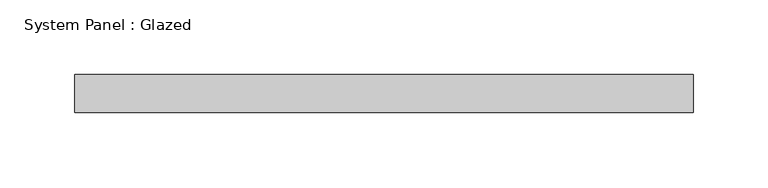
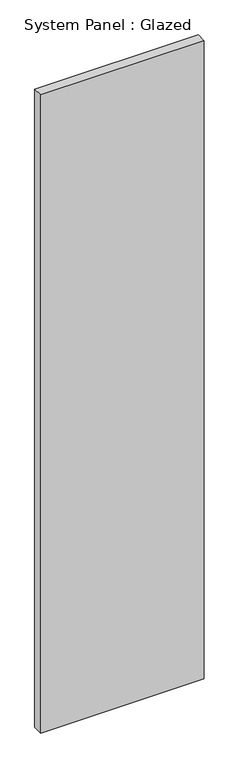
"""IFC4 building model written with IfcOpenShell, lengths in millimetres: plate geometry, System Panel : Glazed."""

from ifc_helpers import new_model, si_unit, origin, origin_with_axes, place, context, project, spatial, polyline, outline, extrude, source, transform, mapped, element, save


def system_panel_glazed_c73a426b(model_context):
    return source(origin(), model_context, "Body", "SweptSolid", [
        extrude(outline(polyline([(206.375, 19.05), (-206.375, 19.05), (-206.375, 44.45), (206.375, 44.45), (206.375, 19.05)])), origin_with_axes(), (0.0, 0.0, 1.0), 1701.8),
    ])


if __name__ == "__main__":
    model = new_model("IFC4")
    model_context = context("Model", 3, world=origin())
    ifc_project = project(units=[si_unit("LENGTHUNIT", "METRE", prefix="MILLI")], contexts=[model_context])
    site = spatial("IfcSite", under=ifc_project)
    building = spatial("IfcBuilding", under=site)
    placement = place(None, origin())
    system_panel_glazed_shape = system_panel_glazed_c73a426b(model_context)
    element("IfcPlate", 1, ObjectType="System Panel : Glazed", at=placement, inside=building, context=model_context, shape_type="MappedRepresentation", body=[
        mapped(system_panel_glazed_shape, transform((0.0, 0.0, 0.0), x_axis=(1.0, 0.0, 0.0), y_axis=(0.0, 1.0, 0.0), z_axis=(0.0, 0.0, 1.0))),
    ])
    save(model, "model.ifc")

# Revit data of these elements
# Type "System Panel : Glazed"
#   Construction Type Id = "GSP4R"
#   Analytic Construction = "1/8 in Pilkington single glazing"
#   Visual Light Transmittance = 0.9
#   Solar Heat Gain Coefficient = 0.86
#   Heat Transfer Coefficient (U) = 1.18115 BTU/(h·ft²·°F)
#   Define Thermal Properties by = 1
# Element 1 (IfcPlate, "System Panel : Glazed")
#   Materials on its faces: "Glass"
# Materials
#   "Glass": class "Glass", colour RGB 0 128 192, transparency 0.75, Description = "Soda Lime Glass", Cost = 0
